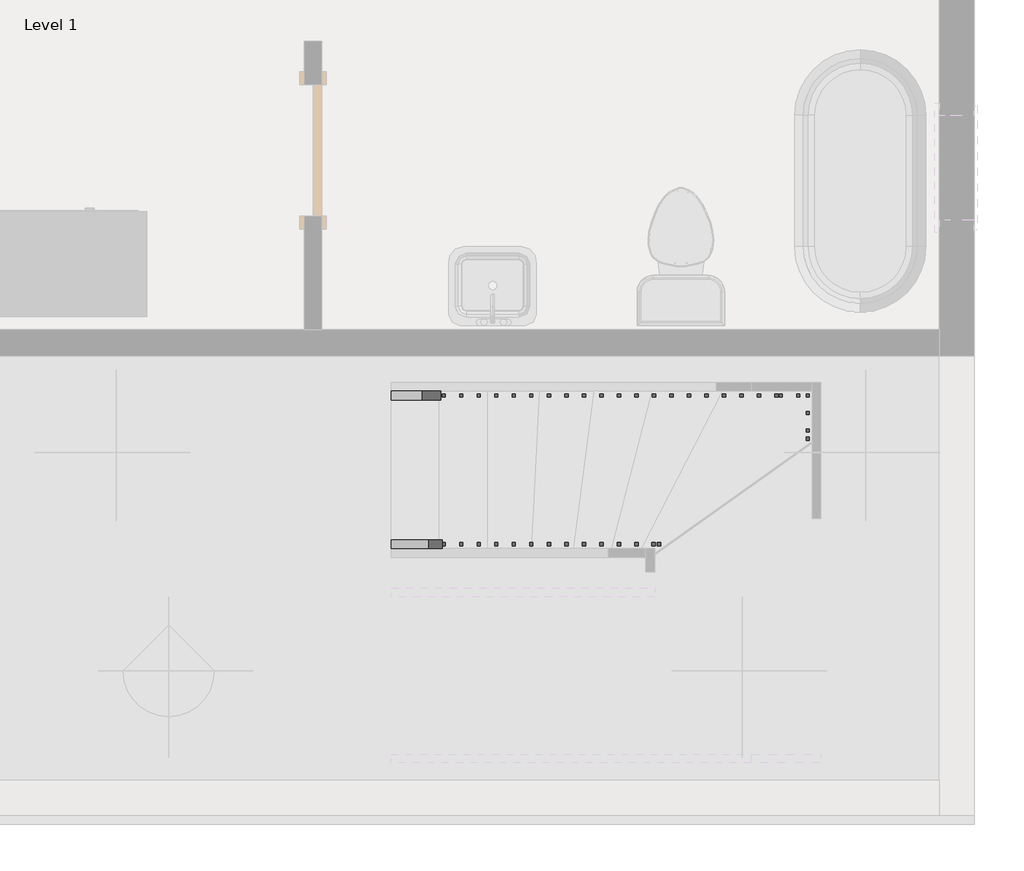
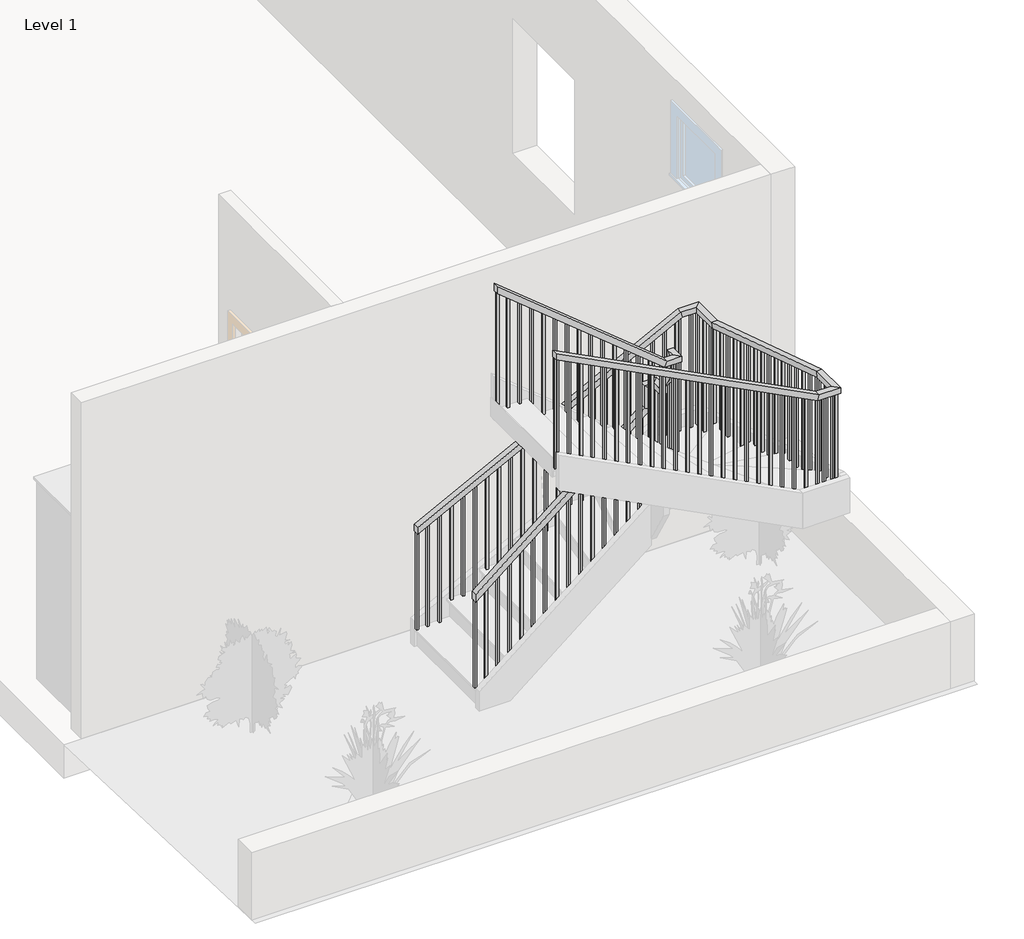
# One storey, part 2 of 3: 2 railings.
"""IFC4 building model written with IfcOpenShell, lengths in millimetres."""

from ifc_helpers import new_model, si_unit, frame, origin, place, context, project, spatial, polyline, outline, extrude, faceted_brep, element, save

model = new_model("IFC4")

# Units and contexts
model_context = context("Model", 3, world=origin())
ifc_project = project(units=[si_unit("LENGTHUNIT", "METRE", prefix="MILLI")], contexts=[model_context])

# Site, building, storey
site = spatial("IfcSite", under=ifc_project)
building = spatial("IfcBuilding", under=site)
storey = spatial("IfcBuildingStorey", under=building, Name="Level 1", Elevation=0.0)

# Railings
placement = place(None, origin())
element("IfcRailing", 1, ObjectType="Handrail - Rectangular", at=placement, inside=storey, context=model_context, shape_type="SolidModel", body=[
    faceted_brep([(3860.8061326, -3864.0192867, 1025.2529681), (3860.8061326, -3864.0192867, 959.7067088), (3860.8061326, -3914.8192867, 959.7067088), (3860.8061326, -3914.8192867, 1025.2529681), (5312.3378245, -3864.0192867, 2208.7848338), (5363.1378245, -3864.0192867, 2184.659247), (5363.1378245, -3914.8192867, 2184.659247), (5312.3378245, -3914.8192867, 2208.7848338), (5312.3378245, -3864.0192867, 2414.6281882), (5363.1378245, -3864.0192867, 2363.8281882), (5363.1378245, -3914.8192867, 2363.8281882), (5312.3378245, -3914.8192867, 2414.6281882), (5439.3378245, -3864.0192867, 2414.6281882), (5439.3378245, -3864.0192867, 2363.8281882), (5388.5378245, -3914.8192867, 2363.8281882), (5388.5378245, -3914.8192867, 2414.6281882), (5439.3378245, -3991.0192867, 2414.6281882), (5439.3378245, -4020.1406205, 2363.8281882), (5388.5378245, -4020.1406205, 2363.8281882), (5388.5378245, -3991.0192867, 2414.6281882), (5439.3378245, -4118.0192867, 2631.5051451), (5439.3378245, -4168.8192867, 2617.7256424), (5388.5378245, -4168.8192867, 2617.7256424), (5388.5378245, -4118.0192867, 2631.5051451), (5439.3378245, -4118.0192867, 2837.3484995), (5439.3378245, -4168.8192867, 2786.5484995), (5388.5378245, -4168.8192867, 2786.5484995), (5388.5378245, -4118.0192867, 2837.3484995), (5439.3378245, -4245.0192867, 2837.3484995), (5439.3378245, -4245.0192867, 2786.5484995), (5388.5378245, -4194.2192867, 2786.5484995), (5388.5378245, -4194.2192867, 2837.3484995), (5312.3378245, -4245.0192867, 2837.3484995), (5294.2524114, -4245.0192867, 2786.5484995), (5294.2524114, -4194.2192867, 2786.5484995), (5312.3378245, -4194.2192867, 2837.3484995), (3860.8061326, -4245.0192867, 4020.8803652), (3860.8061326, -4194.2192867, 4020.8803652), (3860.8061326, -4194.2192867, 3955.3341059), (3860.8061326, -4245.0192867, 3955.3341059)], [[[0, 1, 2, 3]], [[1, 0, 4, 5]], [[2, 1, 5, 6]], [[3, 2, 6, 7]], [[0, 3, 7, 4]], [[5, 4, 8, 9]], [[6, 5, 9, 10]], [[7, 6, 10, 11]], [[4, 7, 11, 8]], [[9, 8, 12, 13]], [[10, 9, 13, 14]], [[11, 10, 14, 15]], [[8, 11, 15, 12]], [[13, 12, 16, 17]], [[14, 13, 17, 18]], [[15, 14, 18, 19]], [[12, 15, 19, 16]], [[17, 16, 20, 21]], [[18, 17, 21, 22]], [[19, 18, 22, 23]], [[16, 19, 23, 20]], [[21, 20, 24, 25]], [[22, 21, 25, 26]], [[23, 22, 26, 27]], [[20, 23, 27, 24]], [[25, 24, 28, 29]], [[26, 25, 29, 30]], [[27, 26, 30, 31]], [[24, 27, 31, 28]], [[29, 28, 32, 33]], [[30, 29, 33, 34]], [[31, 30, 34, 35]], [[28, 31, 35, 32]], [[36, 37, 38, 39]], [[33, 32, 36, 39]], [[34, 33, 39, 38]], [[35, 34, 38, 37]], [[32, 35, 37, 36]]]),
    extrude(outline(polyline([(3866.2231262, 3970.0954681), (3881.7558784, 3951.0454681), (2878.6666667, 3951.0454681), (2878.6666667, 3970.0954681), (3866.2231262, 3970.0954681)])), frame((0.0, -4229.1442867, 0.0), z_axis=(0.0, 1.0, 0.0), x_axis=(0.0, 0.0, 1.0)), (0.0, 0.0, 1.0), 19.05),
    extrude(outline(polyline([(3783.3817813, 4071.6954681), (3798.9145334, 4052.6454681), (2878.6666667, 4052.6454681), (2878.6666667, 4071.6954681), (3783.3817813, 4071.6954681)])), frame((0.0, -4229.1442867, 0.0), z_axis=(0.0, 1.0, 0.0), x_axis=(0.0, 0.0, 1.0)), (0.0, 0.0, 1.0), 19.05),
    extrude(outline(polyline([(3700.5404364, 4173.2954681), (3716.0731885, 4154.2454681), (2709.3333333, 4154.2454681), (2709.3333333, 4173.2954681), (3700.5404364, 4173.2954681)])), frame((0.0, -4229.1442867, 0.0), z_axis=(0.0, 1.0, 0.0), x_axis=(0.0, 0.0, 1.0)), (0.0, 0.0, 1.0), 19.05),
    extrude(outline(polyline([(3617.6990914, 4274.8954681), (3633.2318436, 4255.8454681), (2709.3333333, 4255.8454681), (2709.3333333, 4274.8954681), (3617.6990914, 4274.8954681)])), frame((0.0, -4229.1442867, 0.0), z_axis=(0.0, 1.0, 0.0), x_axis=(0.0, 0.0, 1.0)), (0.0, 0.0, 1.0), 19.05),
    extrude(outline(polyline([(3534.8577465, 4376.4954681), (3550.3904987, 4357.4454681), (2709.3333333, 4357.4454681), (2709.3333333, 4376.4954681), (3534.8577465, 4376.4954681)])), frame((0.0, -4229.1442867, 0.0), z_axis=(0.0, 1.0, 0.0), x_axis=(0.0, 0.0, 1.0)), (0.0, 0.0, 1.0), 19.05),
    extrude(outline(polyline([(3452.0164016, 4478.0954681), (3467.5491538, 4459.0454681), (2540.0, 4459.0454681), (2540.0, 4478.0954681), (3452.0164016, 4478.0954681)])), frame((0.0, -4229.1442867, 0.0), z_axis=(0.0, 1.0, 0.0), x_axis=(0.0, 0.0, 1.0)), (0.0, 0.0, 1.0), 19.05),
    extrude(outline(polyline([(3369.1750567, 4579.6954681), (3384.7078088, 4560.6454681), (2540.0, 4560.6454681), (2540.0, 4579.6954681), (3369.1750567, 4579.6954681)])), frame((0.0, -4229.1442867, 0.0), z_axis=(0.0, 1.0, 0.0), x_axis=(0.0, 0.0, 1.0)), (0.0, 0.0, 1.0), 19.05),
    extrude(outline(polyline([(3286.3337117, 4681.2954681), (3301.8664639, 4662.2454681), (2540.0, 4662.2454681), (2540.0, 4681.2954681), (3286.3337117, 4681.2954681)])), frame((0.0, -4229.1442867, 0.0), z_axis=(0.0, 1.0, 0.0), x_axis=(0.0, 0.0, 1.0)), (0.0, 0.0, 1.0), 19.05),
    extrude(outline(polyline([(3203.4923668, 4782.8954681), (3219.025119, 4763.8454681), (2370.6666667, 4763.8454681), (2370.6666667, 4782.8954681), (3203.4923668, 4782.8954681)])), frame((0.0, -4229.1442867, 0.0), z_axis=(0.0, 1.0, 0.0), x_axis=(0.0, 0.0, 1.0)), (0.0, 0.0, 1.0), 19.05),
    extrude(outline(polyline([(3120.6510219, 4884.4954681), (3136.1837741, 4865.4454681), (2370.6666667, 4865.4454681), (2370.6666667, 4884.4954681), (3120.6510219, 4884.4954681)])), frame((0.0, -4229.1442867, 0.0), z_axis=(0.0, 1.0, 0.0), x_axis=(0.0, 0.0, 1.0)), (0.0, 0.0, 1.0), 19.05),
    extrude(outline(polyline([(3037.809677, 4986.0954681), (3053.3424291, 4967.0454681), (2201.3333333, 4967.0454681), (2201.3333333, 4986.0954681), (3037.809677, 4986.0954681)])), frame((0.0, -4229.1442867, 0.0), z_axis=(0.0, 1.0, 0.0), x_axis=(0.0, 0.0, 1.0)), (0.0, 0.0, 1.0), 19.05),
    extrude(outline(polyline([(2954.9683321, 5087.6954681), (2970.5010842, 5068.6454681), (2201.3333333, 5068.6454681), (2201.3333333, 5087.6954681), (2954.9683321, 5087.6954681)])), frame((0.0, -4229.1442867, 0.0), z_axis=(0.0, 1.0, 0.0), x_axis=(0.0, 0.0, 1.0)), (0.0, 0.0, 1.0), 19.05),
    extrude(outline(polyline([(2872.1269871, 5189.2954681), (2887.6597393, 5170.2454681), (2032.0, 5170.2454681), (2032.0, 5189.2954681), (2872.1269871, 5189.2954681)])), frame((0.0, -4229.1442867, 0.0), z_axis=(0.0, 1.0, 0.0), x_axis=(0.0, 0.0, 1.0)), (0.0, 0.0, 1.0), 19.05),
    extrude(outline(polyline([(2789.2856422, 5290.8954681), (2804.8183944, 5271.8454681), (2032.0, 5271.8454681), (2032.0, 5290.8954681), (2789.2856422, 5290.8954681)])), frame((0.0, -4229.1442867, 0.0), z_axis=(0.0, 1.0, 0.0), x_axis=(0.0, 0.0, 1.0)), (0.0, 0.0, 1.0), 19.05),
    extrude(outline(polyline([(-4116.9301904, 2529.115018), (-4097.8801904, 2496.5834745), (-4097.8801904, 1524.0), (-4116.9301904, 1524.0), (-4116.9301904, 2529.115018)])), frame((5404.4128245, 0.0, 0.0), z_axis=(1.0, 0.0, 0.0), x_axis=(0.0, 1.0, 0.0)), (0.0, 0.0, 1.0), 19.05),
    extrude(outline(polyline([(-4015.3301904, 2355.6134525), (-3996.2801904, 2323.0819089), (-3996.2801904, 1524.0), (-4015.3301904, 1524.0), (-4015.3301904, 2355.6134525)])), frame((5404.4128245, 0.0, 0.0), z_axis=(1.0, 0.0, 0.0), x_axis=(0.0, 1.0, 0.0)), (0.0, 0.0, 1.0), 19.05),
    extrude(outline(polyline([(2127.2519138, 5292.7311326), (2111.7191617, 5273.6811326), (1016.0, 5273.6811326), (1016.0, 5292.7311326), (2127.2519138, 5292.7311326)])), frame((0.0, -3898.9442867, 0.0), z_axis=(0.0, 1.0, 0.0), x_axis=(0.0, 0.0, 1.0)), (0.0, 0.0, 1.0), 19.05),
    extrude(outline(polyline([(2044.4105689, 5191.1311326), (2028.8778167, 5172.0811326), (1016.0, 5172.0811326), (1016.0, 5191.1311326), (2044.4105689, 5191.1311326)])), frame((0.0, -3898.9442867, 0.0), z_axis=(0.0, 1.0, 0.0), x_axis=(0.0, 0.0, 1.0)), (0.0, 0.0, 1.0), 19.05),
    extrude(outline(polyline([(1961.569224, 5089.5311326), (1946.0364718, 5070.4811326), (846.6666667, 5070.4811326), (846.6666667, 5089.5311326), (1961.569224, 5089.5311326)])), frame((0.0, -3898.9442867, 0.0), z_axis=(0.0, 1.0, 0.0), x_axis=(0.0, 0.0, 1.0)), (0.0, 0.0, 1.0), 19.05),
    extrude(outline(polyline([(1878.7278791, 4987.9311326), (1863.1951269, 4968.8811326), (846.6666667, 4968.8811326), (846.6666667, 4987.9311326), (1878.7278791, 4987.9311326)])), frame((0.0, -3898.9442867, 0.0), z_axis=(0.0, 1.0, 0.0), x_axis=(0.0, 0.0, 1.0)), (0.0, 0.0, 1.0), 19.05),
    extrude(outline(polyline([(1795.8865341, 4886.3311326), (1780.353782, 4867.2811326), (677.3333333, 4867.2811326), (677.3333333, 4886.3311326), (1795.8865341, 4886.3311326)])), frame((0.0, -3898.9442867, 0.0), z_axis=(0.0, 1.0, 0.0), x_axis=(0.0, 0.0, 1.0)), (0.0, 0.0, 1.0), 19.05),
    extrude(outline(polyline([(1713.0451892, 4784.7311326), (1697.5124371, 4765.6811326), (677.3333333, 4765.6811326), (677.3333333, 4784.7311326), (1713.0451892, 4784.7311326)])), frame((0.0, -3898.9442867, 0.0), z_axis=(0.0, 1.0, 0.0), x_axis=(0.0, 0.0, 1.0)), (0.0, 0.0, 1.0), 19.05),
    extrude(outline(polyline([(1630.2038443, 4683.1311326), (1614.6710921, 4664.0811326), (508.0, 4664.0811326), (508.0, 4683.1311326), (1630.2038443, 4683.1311326)])), frame((0.0, -3898.9442867, 0.0), z_axis=(0.0, 1.0, 0.0), x_axis=(0.0, 0.0, 1.0)), (0.0, 0.0, 1.0), 19.05),
    extrude(outline(polyline([(1547.3624994, 4581.5311326), (1531.8297472, 4562.4811326), (508.0, 4562.4811326), (508.0, 4581.5311326), (1547.3624994, 4581.5311326)])), frame((0.0, -3898.9442867, 0.0), z_axis=(0.0, 1.0, 0.0), x_axis=(0.0, 0.0, 1.0)), (0.0, 0.0, 1.0), 19.05),
    extrude(outline(polyline([(1464.5211545, 4479.9311326), (1448.9884023, 4460.8811326), (508.0, 4460.8811326), (508.0, 4479.9311326), (1464.5211545, 4479.9311326)])), frame((0.0, -3898.9442867, 0.0), z_axis=(0.0, 1.0, 0.0), x_axis=(0.0, 0.0, 1.0)), (0.0, 0.0, 1.0), 19.05),
    extrude(outline(polyline([(1381.6798095, 4378.3311326), (1366.1470574, 4359.2811326), (338.6666667, 4359.2811326), (338.6666667, 4378.3311326), (1381.6798095, 4378.3311326)])), frame((0.0, -3898.9442867, 0.0), z_axis=(0.0, 1.0, 0.0), x_axis=(0.0, 0.0, 1.0)), (0.0, 0.0, 1.0), 19.05),
    extrude(outline(polyline([(1298.8384646, 4276.7311326), (1283.3057124, 4257.6811326), (338.6666667, 4257.6811326), (338.6666667, 4276.7311326), (1298.8384646, 4276.7311326)])), frame((0.0, -3898.9442867, 0.0), z_axis=(0.0, 1.0, 0.0), x_axis=(0.0, 0.0, 1.0)), (0.0, 0.0, 1.0), 19.05),
    extrude(outline(polyline([(1215.9971197, 4175.1311326), (1200.4643675, 4156.0811326), (338.6666667, 4156.0811326), (338.6666667, 4175.1311326), (1215.9971197, 4175.1311326)])), frame((0.0, -3898.9442867, 0.0), z_axis=(0.0, 1.0, 0.0), x_axis=(0.0, 0.0, 1.0)), (0.0, 0.0, 1.0), 19.05),
    extrude(outline(polyline([(1133.1557748, 4073.5311326), (1117.6230226, 4054.4811326), (169.3333333, 4054.4811326), (169.3333333, 4073.5311326), (1133.1557748, 4073.5311326)])), frame((0.0, -3898.9442867, 0.0), z_axis=(0.0, 1.0, 0.0), x_axis=(0.0, 0.0, 1.0)), (0.0, 0.0, 1.0), 19.05),
    extrude(outline(polyline([(1050.3144298, 3971.9311326), (1034.7816777, 3952.8811326), (169.3333333, 3952.8811326), (169.3333333, 3971.9311326), (1050.3144298, 3971.9311326)])), frame((0.0, -3898.9442867, 0.0), z_axis=(0.0, 1.0, 0.0), x_axis=(0.0, 0.0, 1.0)), (0.0, 0.0, 1.0), 19.05),
    extrude(outline(polyline([(5392.4954681, -4210.0942867), (5392.4954681, -4229.1442867), (5373.4454681, -4229.1442867), (5373.4454681, -4210.0942867), (5392.4954681, -4210.0942867)])), frame((0.0, 0.0, 1862.6666667), z_axis=(0.0, 0.0, 1.0), x_axis=(1.0, 0.0, 0.0)), (0.0, 0.0, 1.0), 923.8818329),
    extrude(outline(polyline([(5404.4128245, -4210.0942867), (5423.4628245, -4210.0942867), (5423.4628245, -4229.1442867), (5404.4128245, -4229.1442867), (5404.4128245, -4210.0942867)])), frame((0.0, 0.0, 1862.6666667), z_axis=(0.0, 0.0, 1.0), x_axis=(1.0, 0.0, 0.0)), (0.0, 0.0, 1.0), 923.8818329),
    extrude(outline(polyline([(5404.4128245, -4195.3083829), (5423.4628245, -4195.3083829), (5423.4628245, -4214.3583829), (5404.4128245, -4214.3583829), (5404.4128245, -4195.3083829)])), frame((0.0, 0.0, 1693.3333333), z_axis=(0.0, 0.0, 1.0), x_axis=(1.0, 0.0, 0.0)), (0.0, 0.0, 1.0), 1093.2151662),
    extrude(outline(polyline([(5404.4128245, -3894.6801904), (5423.4628245, -3894.6801904), (5423.4628245, -3913.7301904), (5404.4128245, -3913.7301904), (5404.4128245, -3894.6801904)])), frame((0.0, 0.0, 1354.6666667), z_axis=(0.0, 0.0, 1.0), x_axis=(1.0, 0.0, 0.0)), (0.0, 0.0, 1.0), 1009.1615215),
    extrude(outline(polyline([(5404.4128245, -3898.9442867), (5404.4128245, -3879.8942867), (5423.4628245, -3879.8942867), (5423.4628245, -3898.9442867), (5404.4128245, -3898.9442867)])), frame((0.0, 0.0, 1185.3333333), z_axis=(0.0, 0.0, 1.0), x_axis=(1.0, 0.0, 0.0)), (0.0, 0.0, 1.0), 1178.4948549),
    extrude(outline(polyline([(5373.4454681, -3898.9442867), (5373.4454681, -3879.8942867), (5392.4954681, -3879.8942867), (5392.4954681, -3898.9442867), (5373.4454681, -3898.9442867)])), frame((0.0, 0.0, 1185.3333333), z_axis=(0.0, 0.0, 1.0), x_axis=(1.0, 0.0, 0.0)), (0.0, 0.0, 1.0), 1178.4948549),
    extrude(outline(polyline([(3939.8013537, 3879.8561326), (3955.3341059, 3860.8061326), (2878.6666667, 3860.8061326), (2878.6666667, 3879.8561326), (3939.8013537, 3879.8561326)])), frame((0.0, -4229.1442867, 0.0), z_axis=(0.0, 1.0, 0.0), x_axis=(0.0, 0.0, 1.0)), (0.0, 0.0, 1.0), 19.05),
    extrude(outline(polyline([(975.239461, 3879.8561326), (959.7067088, 3860.8061326), (169.3333333, 3860.8061326), (169.3333333, 3879.8561326), (975.239461, 3879.8561326)])), frame((0.0, -3898.9442867, 0.0), z_axis=(0.0, 1.0, 0.0), x_axis=(0.0, 0.0, 1.0)), (0.0, 0.0, 1.0), 19.05),
])
element("IfcRailing", 2, ObjectType="Handrail - Rectangular", at=placement, inside=storey, context=model_context, shape_type="SolidModel", body=[
    faceted_brep([(3860.8061326, -3000.4192867, 1109.0771751), (3860.8061326, -3000.4192867, 1051.9280057), (3860.8061326, -3051.2192867, 1051.9280057), (3860.8061326, -3051.2192867, 1109.0771751), (6120.7879891, -3000.4192867, 2273.7644996), (6133.1080404, -3000.4192867, 2222.9644996), (6133.1080404, -3051.2192867, 2222.9644996), (6120.7879891, -3051.2192867, 2273.7644996), (6302.9378245, -3000.4192867, 2273.7644996), (6302.9378245, -3000.4192867, 2222.9644996), (6252.1378245, -3051.2192867, 2222.9644996), (6252.1378245, -3051.2192867, 2273.7644996), (6302.9378245, -3277.5732393, 2273.7644996), (6302.9378245, -3285.5238154, 2222.9644996), (6252.1378245, -3285.5238154, 2222.9644996), (6252.1378245, -3277.5732393, 2273.7644996), (6302.9378245, -4831.4653341, 2772.3688337), (6302.9378245, -4839.4159102, 2721.5688337), (6252.1378245, -4839.4159102, 2721.5688337), (6252.1378245, -4831.4653341, 2772.3688337), (6302.9378245, -5108.6192867, 2772.3688337), (6302.9378245, -5108.6192867, 2721.5688337), (6252.1378245, -5057.8192867, 2721.5688337), (6252.1378245, -5057.8192867, 2772.3688337), (6120.7879891, -5108.6192867, 2772.3688337), (6108.4679378, -5108.6192867, 2721.5688337), (6108.4679378, -5057.8192867, 2721.5688337), (6120.7879891, -5057.8192867, 2772.3688337), (3860.8061326, -5108.6192867, 3937.0561582), (3860.8061326, -5057.8192867, 3937.0561582), (3860.8061326, -5057.8192867, 3879.9069889), (3860.8061326, -5108.6192867, 3879.9069889)], [[[0, 1, 2, 3]], [[1, 0, 4, 5]], [[2, 1, 5, 6]], [[3, 2, 6, 7]], [[0, 3, 7, 4]], [[5, 4, 8, 9]], [[6, 5, 9, 10]], [[7, 6, 10, 11]], [[4, 7, 11, 8]], [[9, 8, 12, 13]], [[10, 9, 13, 14]], [[11, 10, 14, 15]], [[8, 11, 15, 12]], [[13, 12, 16, 17]], [[14, 13, 17, 18]], [[15, 14, 18, 19]], [[12, 15, 19, 16]], [[17, 16, 20, 21]], [[18, 17, 21, 22]], [[19, 18, 22, 23]], [[16, 19, 23, 20]], [[21, 20, 24, 25]], [[22, 21, 25, 26]], [[23, 22, 26, 27]], [[20, 23, 27, 24]], [[28, 29, 30, 31]], [[25, 24, 28, 31]], [[26, 25, 31, 30]], [[27, 26, 30, 29]], [[24, 27, 29, 28]]]),
    extrude(outline(polyline([(3872.0443296, 3876.0629891), (2878.6666667, 3876.0629891), (2878.6666667, 3895.1129891), (3862.2268642, 3895.1129891), (3872.0443296, 3876.0629891)])), frame((0.0, -5092.7442867, 0.0), z_axis=(0.0, 1.0, 0.0), x_axis=(0.0, 0.0, 1.0)), (0.0, 0.0, 1.0), 19.05),
    extrude(outline(polyline([(3819.6845145, 3977.6629891), (2878.6666667, 3977.6629891), (2878.6666667, 3996.7129891), (3809.8670491, 3996.7129891), (3819.6845145, 3977.6629891)])), frame((0.0, -5092.7442867, 0.0), z_axis=(0.0, 1.0, 0.0), x_axis=(0.0, 0.0, 1.0)), (0.0, 0.0, 1.0), 19.05),
    extrude(outline(polyline([(3767.3246993, 4079.2629891), (2878.6666667, 4079.2629891), (2878.6666667, 4098.3129891), (3757.507234, 4098.3129891), (3767.3246993, 4079.2629891)])), frame((0.0, -5092.7442867, 0.0), z_axis=(0.0, 1.0, 0.0), x_axis=(0.0, 0.0, 1.0)), (0.0, 0.0, 1.0), 19.05),
    extrude(outline(polyline([(3714.9648842, 4180.8629891), (2709.3333333, 4180.8629891), (2709.3333333, 4199.9129891), (3705.1474189, 4199.9129891), (3714.9648842, 4180.8629891)])), frame((0.0, -5092.7442867, 0.0), z_axis=(0.0, 1.0, 0.0), x_axis=(0.0, 0.0, 1.0)), (0.0, 0.0, 1.0), 19.05),
    extrude(outline(polyline([(3662.6050691, 4282.4629891), (2709.3333333, 4282.4629891), (2709.3333333, 4301.5129891), (3652.7876038, 4301.5129891), (3662.6050691, 4282.4629891)])), frame((0.0, -5092.7442867, 0.0), z_axis=(0.0, 1.0, 0.0), x_axis=(0.0, 0.0, 1.0)), (0.0, 0.0, 1.0), 19.05),
    extrude(outline(polyline([(3610.245254, 4384.0629891), (2709.3333333, 4384.0629891), (2709.3333333, 4403.1129891), (3600.4277887, 4403.1129891), (3610.245254, 4384.0629891)])), frame((0.0, -5092.7442867, 0.0), z_axis=(0.0, 1.0, 0.0), x_axis=(0.0, 0.0, 1.0)), (0.0, 0.0, 1.0), 19.05),
    extrude(outline(polyline([(3557.8854389, 4485.6629891), (2540.0, 4485.6629891), (2540.0, 4504.7129891), (3548.0679735, 4504.7129891), (3557.8854389, 4485.6629891)])), frame((0.0, -5092.7442867, 0.0), z_axis=(0.0, 1.0, 0.0), x_axis=(0.0, 0.0, 1.0)), (0.0, 0.0, 1.0), 19.05),
    extrude(outline(polyline([(3505.5256238, 4587.2629891), (2540.0, 4587.2629891), (2540.0, 4606.3129891), (3495.7081584, 4606.3129891), (3505.5256238, 4587.2629891)])), frame((0.0, -5092.7442867, 0.0), z_axis=(0.0, 1.0, 0.0), x_axis=(0.0, 0.0, 1.0)), (0.0, 0.0, 1.0), 19.05),
    extrude(outline(polyline([(3453.1658086, 4688.8629891), (2540.0, 4688.8629891), (2540.0, 4707.9129891), (3443.3483433, 4707.9129891), (3453.1658086, 4688.8629891)])), frame((0.0, -5092.7442867, 0.0), z_axis=(0.0, 1.0, 0.0), x_axis=(0.0, 0.0, 1.0)), (0.0, 0.0, 1.0), 19.05),
    extrude(outline(polyline([(3400.8059935, 4790.4629891), (2370.6666667, 4790.4629891), (2370.6666667, 4809.5129891), (3390.9885282, 4809.5129891), (3400.8059935, 4790.4629891)])), frame((0.0, -5092.7442867, 0.0), z_axis=(0.0, 1.0, 0.0), x_axis=(0.0, 0.0, 1.0)), (0.0, 0.0, 1.0), 19.05),
    extrude(outline(polyline([(3348.4461784, 4892.0629891), (2370.6666667, 4892.0629891), (2370.6666667, 4911.1129891), (3338.6287131, 4911.1129891), (3348.4461784, 4892.0629891)])), frame((0.0, -5092.7442867, 0.0), z_axis=(0.0, 1.0, 0.0), x_axis=(0.0, 0.0, 1.0)), (0.0, 0.0, 1.0), 19.05),
    extrude(outline(polyline([(3296.0863633, 4993.6629891), (2370.6666667, 4993.6629891), (2370.6666667, 5012.7129891), (3286.268898, 5012.7129891), (3296.0863633, 4993.6629891)])), frame((0.0, -5092.7442867, 0.0), z_axis=(0.0, 1.0, 0.0), x_axis=(0.0, 0.0, 1.0)), (0.0, 0.0, 1.0), 19.05),
    extrude(outline(polyline([(3243.7265482, 5095.2629891), (2201.3333333, 5095.2629891), (2201.3333333, 5114.3129891), (3233.9090828, 5114.3129891), (3243.7265482, 5095.2629891)])), frame((0.0, -5092.7442867, 0.0), z_axis=(0.0, 1.0, 0.0), x_axis=(0.0, 0.0, 1.0)), (0.0, 0.0, 1.0), 19.05),
    extrude(outline(polyline([(3191.3667331, 5196.8629891), (2201.3333333, 5196.8629891), (2201.3333333, 5215.9129891), (3181.5492677, 5215.9129891), (3191.3667331, 5196.8629891)])), frame((0.0, -5092.7442867, 0.0), z_axis=(0.0, 1.0, 0.0), x_axis=(0.0, 0.0, 1.0)), (0.0, 0.0, 1.0), 19.05),
    extrude(outline(polyline([(3139.0069179, 5298.4629891), (2201.3333333, 5298.4629891), (2201.3333333, 5317.5129891), (3129.1894526, 5317.5129891), (3139.0069179, 5298.4629891)])), frame((0.0, -5092.7442867, 0.0), z_axis=(0.0, 1.0, 0.0), x_axis=(0.0, 0.0, 1.0)), (0.0, 0.0, 1.0), 19.05),
    extrude(outline(polyline([(3086.6471028, 5400.0629891), (2032.0, 5400.0629891), (2032.0, 5419.1129891), (3076.8296375, 5419.1129891), (3086.6471028, 5400.0629891)])), frame((0.0, -5092.7442867, 0.0), z_axis=(0.0, 1.0, 0.0), x_axis=(0.0, 0.0, 1.0)), (0.0, 0.0, 1.0), 19.05),
    extrude(outline(polyline([(3034.2872877, 5501.6629891), (2032.0, 5501.6629891), (2032.0, 5520.7129891), (3024.4698224, 5520.7129891), (3034.2872877, 5501.6629891)])), frame((0.0, -5092.7442867, 0.0), z_axis=(0.0, 1.0, 0.0), x_axis=(0.0, 0.0, 1.0)), (0.0, 0.0, 1.0), 19.05),
    extrude(outline(polyline([(2981.9274726, 5603.2629891), (2032.0, 5603.2629891), (2032.0, 5622.3129891), (2972.1100073, 5622.3129891), (2981.9274726, 5603.2629891)])), frame((0.0, -5092.7442867, 0.0), z_axis=(0.0, 1.0, 0.0), x_axis=(0.0, 0.0, 1.0)), (0.0, 0.0, 1.0), 19.05),
    extrude(outline(polyline([(2929.5676575, 5704.8629891), (2032.0, 5704.8629891), (2032.0, 5723.9129891), (2919.7501921, 5723.9129891), (2929.5676575, 5704.8629891)])), frame((0.0, -5092.7442867, 0.0), z_axis=(0.0, 1.0, 0.0), x_axis=(0.0, 0.0, 1.0)), (0.0, 0.0, 1.0), 19.05),
    extrude(outline(polyline([(2877.2078424, 5806.4629891), (1862.6666667, 5806.4629891), (1862.6666667, 5825.5129891), (2867.390377, 5825.5129891), (2877.2078424, 5806.4629891)])), frame((0.0, -5092.7442867, 0.0), z_axis=(0.0, 1.0, 0.0), x_axis=(0.0, 0.0, 1.0)), (0.0, 0.0, 1.0), 19.05),
    extrude(outline(polyline([(2824.8480272, 5908.0629891), (1862.6666667, 5908.0629891), (1862.6666667, 5927.1129891), (2815.0305619, 5927.1129891), (2824.8480272, 5908.0629891)])), frame((0.0, -5092.7442867, 0.0), z_axis=(0.0, 1.0, 0.0), x_axis=(0.0, 0.0, 1.0)), (0.0, 0.0, 1.0), 19.05),
    extrude(outline(polyline([(2772.4882121, 6009.6629891), (1862.6666667, 6009.6629891), (1862.6666667, 6028.7129891), (2762.6707468, 6028.7129891), (2772.4882121, 6009.6629891)])), frame((0.0, -5092.7442867, 0.0), z_axis=(0.0, 1.0, 0.0), x_axis=(0.0, 0.0, 1.0)), (0.0, 0.0, 1.0), 19.05),
    extrude(outline(polyline([(6185.4628245, -5092.7442867), (6166.4128245, -5092.7442867), (6166.4128245, -5073.6942867), (6185.4628245, -5073.6942867), (6185.4628245, -5092.7442867)])), frame((0.0, 0.0, 1862.6666667), z_axis=(0.0, 0.0, 1.0), x_axis=(1.0, 0.0, 0.0)), (0.0, 0.0, 1.0), 858.902167),
    extrude(outline(polyline([(6287.0628245, -5025.1403341), (6287.0628245, -5044.1903341), (6268.0128245, -5044.1903341), (6268.0128245, -5025.1403341), (6287.0628245, -5025.1403341)])), frame((0.0, 0.0, 1862.6666667), z_axis=(0.0, 0.0, 1.0), x_axis=(1.0, 0.0, 0.0)), (0.0, 0.0, 1.0), 858.902167),
    extrude(outline(polyline([(6287.0628245, -4923.5403341), (6287.0628245, -4942.5903341), (6268.0128245, -4942.5903341), (6268.0128245, -4923.5403341), (6287.0628245, -4923.5403341)])), frame((0.0, 0.0, 1862.6666667), z_axis=(0.0, 0.0, 1.0), x_axis=(1.0, 0.0, 0.0)), (0.0, 0.0, 1.0), 858.902167),
    extrude(outline(polyline([(-4792.0482393, 2706.3697564), (-4792.0482393, 1693.3333333), (-4811.0982393, 1693.3333333), (-4811.0982393, 2712.4824155), (-4792.0482393, 2706.3697564)])), frame((6268.0128245, 0.0, 0.0), z_axis=(1.0, 0.0, 0.0), x_axis=(0.0, 1.0, 0.0)), (0.0, 0.0, 1.0), 19.05),
    extrude(outline(polyline([(-4690.4482393, 2673.7689082), (-4690.4482393, 1693.3333333), (-4709.4982393, 1693.3333333), (-4709.4982393, 2679.8815673), (-4690.4482393, 2673.7689082)])), frame((6268.0128245, 0.0, 0.0), z_axis=(1.0, 0.0, 0.0), x_axis=(0.0, 1.0, 0.0)), (0.0, 0.0, 1.0), 19.05),
    extrude(outline(polyline([(-4588.8482393, 2641.16806), (-4588.8482393, 1693.3333333), (-4607.8982393, 1693.3333333), (-4607.8982393, 2647.280719), (-4588.8482393, 2641.16806)])), frame((6268.0128245, 0.0, 0.0), z_axis=(1.0, 0.0, 0.0), x_axis=(0.0, 1.0, 0.0)), (0.0, 0.0, 1.0), 19.05),
    extrude(outline(polyline([(-4487.2482393, 2608.5672118), (-4487.2482393, 1693.3333333), (-4506.2982393, 1693.3333333), (-4506.2982393, 2614.6798708), (-4487.2482393, 2608.5672118)])), frame((6268.0128245, 0.0, 0.0), z_axis=(1.0, 0.0, 0.0), x_axis=(0.0, 1.0, 0.0)), (0.0, 0.0, 1.0), 19.05),
    extrude(outline(polyline([(-4385.6482393, 2575.9663635), (-4385.6482393, 1693.3333333), (-4404.6982393, 1693.3333333), (-4404.6982393, 2582.0790226), (-4385.6482393, 2575.9663635)])), frame((6268.0128245, 0.0, 0.0), z_axis=(1.0, 0.0, 0.0), x_axis=(0.0, 1.0, 0.0)), (0.0, 0.0, 1.0), 19.05),
    extrude(outline(polyline([(-4284.0482393, 2543.3655153), (-4284.0482393, 1693.3333333), (-4303.0982393, 1693.3333333), (-4303.0982393, 2549.4781744), (-4284.0482393, 2543.3655153)])), frame((6268.0128245, 0.0, 0.0), z_axis=(1.0, 0.0, 0.0), x_axis=(0.0, 1.0, 0.0)), (0.0, 0.0, 1.0), 19.05),
    extrude(outline(polyline([(-4182.4482393, 2510.7646671), (-4182.4482393, 1524.0), (-4201.4982393, 1524.0), (-4201.4982393, 2516.8773261), (-4182.4482393, 2510.7646671)])), frame((6268.0128245, 0.0, 0.0), z_axis=(1.0, 0.0, 0.0), x_axis=(0.0, 1.0, 0.0)), (0.0, 0.0, 1.0), 19.05),
    extrude(outline(polyline([(-4080.8482393, 2478.1638189), (-4080.8482393, 1524.0), (-4099.8982393, 1524.0), (-4099.8982393, 2484.2764779), (-4080.8482393, 2478.1638189)])), frame((6268.0128245, 0.0, 0.0), z_axis=(1.0, 0.0, 0.0), x_axis=(0.0, 1.0, 0.0)), (0.0, 0.0, 1.0), 19.05),
    extrude(outline(polyline([(-3979.2482393, 2445.5629706), (-3979.2482393, 1524.0), (-3998.2982393, 1524.0), (-3998.2982393, 2451.6756297), (-3979.2482393, 2445.5629706)])), frame((6268.0128245, 0.0, 0.0), z_axis=(1.0, 0.0, 0.0), x_axis=(0.0, 1.0, 0.0)), (0.0, 0.0, 1.0), 19.05),
    extrude(outline(polyline([(-3877.6482393, 2412.9621224), (-3877.6482393, 1524.0), (-3896.6982393, 1524.0), (-3896.6982393, 2419.0747814), (-3877.6482393, 2412.9621224)])), frame((6268.0128245, 0.0, 0.0), z_axis=(1.0, 0.0, 0.0), x_axis=(0.0, 1.0, 0.0)), (0.0, 0.0, 1.0), 19.05),
    extrude(outline(polyline([(-3776.0482393, 2380.3612742), (-3776.0482393, 1354.6666667), (-3795.0982393, 1354.6666667), (-3795.0982393, 2386.4739332), (-3776.0482393, 2380.3612742)])), frame((6268.0128245, 0.0, 0.0), z_axis=(1.0, 0.0, 0.0), x_axis=(0.0, 1.0, 0.0)), (0.0, 0.0, 1.0), 19.05),
    extrude(outline(polyline([(-3674.4482393, 2347.7604259), (-3674.4482393, 1354.6666667), (-3693.4982393, 1354.6666667), (-3693.4982393, 2353.873085), (-3674.4482393, 2347.7604259)])), frame((6268.0128245, 0.0, 0.0), z_axis=(1.0, 0.0, 0.0), x_axis=(0.0, 1.0, 0.0)), (0.0, 0.0, 1.0), 19.05),
    extrude(outline(polyline([(-3572.8482393, 2315.1595777), (-3572.8482393, 1354.6666667), (-3591.8982393, 1354.6666667), (-3591.8982393, 2321.2722368), (-3572.8482393, 2315.1595777)])), frame((6268.0128245, 0.0, 0.0), z_axis=(1.0, 0.0, 0.0), x_axis=(0.0, 1.0, 0.0)), (0.0, 0.0, 1.0), 19.05),
    extrude(outline(polyline([(-3471.2482393, 2282.5587295), (-3471.2482393, 1354.6666667), (-3490.2982393, 1354.6666667), (-3490.2982393, 2288.6713885), (-3471.2482393, 2282.5587295)])), frame((6268.0128245, 0.0, 0.0), z_axis=(1.0, 0.0, 0.0), x_axis=(0.0, 1.0, 0.0)), (0.0, 0.0, 1.0), 19.05),
    extrude(outline(polyline([(-3369.6482393, 2249.9578813), (-3369.6482393, 1354.6666667), (-3388.6982393, 1354.6666667), (-3388.6982393, 2256.0705403), (-3369.6482393, 2249.9578813)])), frame((6268.0128245, 0.0, 0.0), z_axis=(1.0, 0.0, 0.0), x_axis=(0.0, 1.0, 0.0)), (0.0, 0.0, 1.0), 19.05),
    extrude(outline(polyline([(6287.0628245, -3219.4942867), (6287.0628245, -3238.5442867), (6268.0128245, -3238.5442867), (6268.0128245, -3219.4942867), (6287.0628245, -3219.4942867)])), frame((0.0, 0.0, 1185.3333333), z_axis=(0.0, 0.0, 1.0), x_axis=(1.0, 0.0, 0.0)), (0.0, 0.0, 1.0), 1037.6311663),
    extrude(outline(polyline([(6287.0628245, -3117.8942867), (6287.0628245, -3136.9442867), (6268.0128245, -3136.9442867), (6268.0128245, -3117.8942867), (6287.0628245, -3117.8942867)])), frame((0.0, 0.0, 1185.3333333), z_axis=(0.0, 0.0, 1.0), x_axis=(1.0, 0.0, 0.0)), (0.0, 0.0, 1.0), 1037.6311663),
    extrude(outline(polyline([(6212.8629891, -3016.2942867), (6231.9129891, -3016.2942867), (6231.9129891, -3035.3442867), (6212.8629891, -3035.3442867), (6212.8629891, -3016.2942867)])), frame((0.0, 0.0, 1185.3333333), z_axis=(0.0, 0.0, 1.0), x_axis=(1.0, 0.0, 0.0)), (0.0, 0.0, 1.0), 1037.6311663),
    extrude(outline(polyline([(2198.9352056, 6086.4811326), (1185.3333333, 6086.4811326), (1185.3333333, 6105.5311326), (2208.752671, 6105.5311326), (2198.9352056, 6086.4811326)])), frame((0.0, -3035.3442867, 0.0), z_axis=(0.0, 1.0, 0.0), x_axis=(0.0, 0.0, 1.0)), (0.0, 0.0, 1.0), 19.05),
    extrude(outline(polyline([(2146.5753905, 5984.8811326), (1185.3333333, 5984.8811326), (1185.3333333, 6003.9311326), (2156.3928558, 6003.9311326), (2146.5753905, 5984.8811326)])), frame((0.0, -3035.3442867, 0.0), z_axis=(0.0, 1.0, 0.0), x_axis=(0.0, 0.0, 1.0)), (0.0, 0.0, 1.0), 19.05),
    extrude(outline(polyline([(2094.2155754, 5883.2811326), (1185.3333333, 5883.2811326), (1185.3333333, 5902.3311326), (2104.0330407, 5902.3311326), (2094.2155754, 5883.2811326)])), frame((0.0, -3035.3442867, 0.0), z_axis=(0.0, 1.0, 0.0), x_axis=(0.0, 0.0, 1.0)), (0.0, 0.0, 1.0), 19.05),
    extrude(outline(polyline([(2041.8557603, 5781.6811326), (1185.3333333, 5781.6811326), (1185.3333333, 5800.7311326), (2051.6732256, 5800.7311326), (2041.8557603, 5781.6811326)])), frame((0.0, -3035.3442867, 0.0), z_axis=(0.0, 1.0, 0.0), x_axis=(0.0, 0.0, 1.0)), (0.0, 0.0, 1.0), 19.05),
    extrude(outline(polyline([(1989.4959452, 5680.0811326), (1016.0, 5680.0811326), (1016.0, 5699.1311326), (1999.3134105, 5699.1311326), (1989.4959452, 5680.0811326)])), frame((0.0, -3035.3442867, 0.0), z_axis=(0.0, 1.0, 0.0), x_axis=(0.0, 0.0, 1.0)), (0.0, 0.0, 1.0), 19.05),
    extrude(outline(polyline([(1937.13613, 5578.4811326), (1016.0, 5578.4811326), (1016.0, 5597.5311326), (1946.9535954, 5597.5311326), (1937.13613, 5578.4811326)])), frame((0.0, -3035.3442867, 0.0), z_axis=(0.0, 1.0, 0.0), x_axis=(0.0, 0.0, 1.0)), (0.0, 0.0, 1.0), 19.05),
    extrude(outline(polyline([(1884.7763149, 5476.8811326), (1016.0, 5476.8811326), (1016.0, 5495.9311326), (1894.5937803, 5495.9311326), (1884.7763149, 5476.8811326)])), frame((0.0, -3035.3442867, 0.0), z_axis=(0.0, 1.0, 0.0), x_axis=(0.0, 0.0, 1.0)), (0.0, 0.0, 1.0), 19.05),
    extrude(outline(polyline([(1832.4164998, 5375.2811326), (1016.0, 5375.2811326), (1016.0, 5394.3311326), (1842.2339651, 5394.3311326), (1832.4164998, 5375.2811326)])), frame((0.0, -3035.3442867, 0.0), z_axis=(0.0, 1.0, 0.0), x_axis=(0.0, 0.0, 1.0)), (0.0, 0.0, 1.0), 19.05),
    extrude(outline(polyline([(1780.0566847, 5273.6811326), (846.6666667, 5273.6811326), (846.6666667, 5292.7311326), (1789.87415, 5292.7311326), (1780.0566847, 5273.6811326)])), frame((0.0, -3035.3442867, 0.0), z_axis=(0.0, 1.0, 0.0), x_axis=(0.0, 0.0, 1.0)), (0.0, 0.0, 1.0), 19.05),
    extrude(outline(polyline([(1727.6968696, 5172.0811326), (846.6666667, 5172.0811326), (846.6666667, 5191.1311326), (1737.5143349, 5191.1311326), (1727.6968696, 5172.0811326)])), frame((0.0, -3035.3442867, 0.0), z_axis=(0.0, 1.0, 0.0), x_axis=(0.0, 0.0, 1.0)), (0.0, 0.0, 1.0), 19.05),
    extrude(outline(polyline([(1675.3370545, 5070.4811326), (846.6666667, 5070.4811326), (846.6666667, 5089.5311326), (1685.1545198, 5089.5311326), (1675.3370545, 5070.4811326)])), frame((0.0, -3035.3442867, 0.0), z_axis=(0.0, 1.0, 0.0), x_axis=(0.0, 0.0, 1.0)), (0.0, 0.0, 1.0), 19.05),
    extrude(outline(polyline([(1622.9772393, 4968.8811326), (677.3333333, 4968.8811326), (677.3333333, 4987.9311326), (1632.7947047, 4987.9311326), (1622.9772393, 4968.8811326)])), frame((0.0, -3035.3442867, 0.0), z_axis=(0.0, 1.0, 0.0), x_axis=(0.0, 0.0, 1.0)), (0.0, 0.0, 1.0), 19.05),
    extrude(outline(polyline([(1570.6174242, 4867.2811326), (677.3333333, 4867.2811326), (677.3333333, 4886.3311326), (1580.4348896, 4886.3311326), (1570.6174242, 4867.2811326)])), frame((0.0, -3035.3442867, 0.0), z_axis=(0.0, 1.0, 0.0), x_axis=(0.0, 0.0, 1.0)), (0.0, 0.0, 1.0), 19.05),
    extrude(outline(polyline([(1518.2576091, 4765.6811326), (677.3333333, 4765.6811326), (677.3333333, 4784.7311326), (1528.0750744, 4784.7311326), (1518.2576091, 4765.6811326)])), frame((0.0, -3035.3442867, 0.0), z_axis=(0.0, 1.0, 0.0), x_axis=(0.0, 0.0, 1.0)), (0.0, 0.0, 1.0), 19.05),
    extrude(outline(polyline([(1465.897794, 4664.0811326), (508.0, 4664.0811326), (508.0, 4683.1311326), (1475.7152593, 4683.1311326), (1465.897794, 4664.0811326)])), frame((0.0, -3035.3442867, 0.0), z_axis=(0.0, 1.0, 0.0), x_axis=(0.0, 0.0, 1.0)), (0.0, 0.0, 1.0), 19.05),
    extrude(outline(polyline([(1413.5379789, 4562.4811326), (508.0, 4562.4811326), (508.0, 4581.5311326), (1423.3554442, 4581.5311326), (1413.5379789, 4562.4811326)])), frame((0.0, -3035.3442867, 0.0), z_axis=(0.0, 1.0, 0.0), x_axis=(0.0, 0.0, 1.0)), (0.0, 0.0, 1.0), 19.05),
    extrude(outline(polyline([(1361.1781638, 4460.8811326), (508.0, 4460.8811326), (508.0, 4479.9311326), (1370.9956291, 4479.9311326), (1361.1781638, 4460.8811326)])), frame((0.0, -3035.3442867, 0.0), z_axis=(0.0, 1.0, 0.0), x_axis=(0.0, 0.0, 1.0)), (0.0, 0.0, 1.0), 19.05),
    extrude(outline(polyline([(1308.8183486, 4359.2811326), (338.6666667, 4359.2811326), (338.6666667, 4378.3311326), (1318.635814, 4378.3311326), (1308.8183486, 4359.2811326)])), frame((0.0, -3035.3442867, 0.0), z_axis=(0.0, 1.0, 0.0), x_axis=(0.0, 0.0, 1.0)), (0.0, 0.0, 1.0), 19.05),
    extrude(outline(polyline([(1256.4585335, 4257.6811326), (338.6666667, 4257.6811326), (338.6666667, 4276.7311326), (1266.2759989, 4276.7311326), (1256.4585335, 4257.6811326)])), frame((0.0, -3035.3442867, 0.0), z_axis=(0.0, 1.0, 0.0), x_axis=(0.0, 0.0, 1.0)), (0.0, 0.0, 1.0), 19.05),
    extrude(outline(polyline([(1204.0987184, 4156.0811326), (338.6666667, 4156.0811326), (338.6666667, 4175.1311326), (1213.9161837, 4175.1311326), (1204.0987184, 4156.0811326)])), frame((0.0, -3035.3442867, 0.0), z_axis=(0.0, 1.0, 0.0), x_axis=(0.0, 0.0, 1.0)), (0.0, 0.0, 1.0), 19.05),
    extrude(outline(polyline([(1151.7389033, 4054.4811326), (169.3333333, 4054.4811326), (169.3333333, 4073.5311326), (1161.5563686, 4073.5311326), (1151.7389033, 4054.4811326)])), frame((0.0, -3035.3442867, 0.0), z_axis=(0.0, 1.0, 0.0), x_axis=(0.0, 0.0, 1.0)), (0.0, 0.0, 1.0), 19.05),
    extrude(outline(polyline([(1099.3790882, 3952.8811326), (169.3333333, 3952.8811326), (169.3333333, 3971.9311326), (1109.1965535, 3971.9311326), (1099.3790882, 3952.8811326)])), frame((0.0, -3035.3442867, 0.0), z_axis=(0.0, 1.0, 0.0), x_axis=(0.0, 0.0, 1.0)), (0.0, 0.0, 1.0), 19.05),
    extrude(outline(polyline([(6130.3129891, -5092.7442867), (6111.2629891, -5092.7442867), (6111.2629891, -5073.6942867), (6130.3129891, -5073.6942867), (6130.3129891, -5092.7442867)])), frame((0.0, 0.0, 1862.6666667), z_axis=(0.0, 0.0, 1.0), x_axis=(1.0, 0.0, 0.0)), (0.0, 0.0, 1.0), 858.902167),
    extrude(outline(polyline([(6287.0628245, -5073.6942867), (6287.0628245, -5092.7442867), (6268.0128245, -5092.7442867), (6268.0128245, -5073.6942867), (6287.0628245, -5073.6942867)])), frame((0.0, 0.0, 1862.6666667), z_axis=(0.0, 0.0, 1.0), x_axis=(1.0, 0.0, 0.0)), (0.0, 0.0, 1.0), 858.902167),
    extrude(outline(polyline([(-4821.9403341, 2715.9613671), (-4821.9403341, 1862.6666667), (-4840.9903341, 1862.6666667), (-4840.9903341, 2722.0740262), (-4821.9403341, 2715.9613671)])), frame((6268.0128245, 0.0, 0.0), z_axis=(1.0, 0.0, 0.0), x_axis=(0.0, 1.0, 0.0)), (0.0, 0.0, 1.0), 19.05),
    extrude(outline(polyline([(6287.0628245, -3268.0482393), (6287.0628245, -3287.0982393), (6268.0128245, -3287.0982393), (6268.0128245, -3268.0482393), (6287.0628245, -3268.0482393)])), frame((0.0, 0.0, 1185.3333333), z_axis=(0.0, 0.0, 1.0), x_axis=(1.0, 0.0, 0.0)), (0.0, 0.0, 1.0), 1037.6311663),
    extrude(outline(polyline([(6268.0128245, -3016.2942867), (6287.0628245, -3016.2942867), (6287.0628245, -3035.3442867), (6268.0128245, -3035.3442867), (6268.0128245, -3016.2942867)])), frame((0.0, 0.0, 1185.3333333), z_axis=(0.0, 0.0, 1.0), x_axis=(1.0, 0.0, 0.0)), (0.0, 0.0, 1.0), 1037.6311663),
    extrude(outline(polyline([(2211.7065976, 6111.2629891), (1185.3333333, 6111.2629891), (1185.3333333, 6130.3129891), (2221.5240629, 6130.3129891), (2211.7065976, 6111.2629891)])), frame((0.0, -3035.3442867, 0.0), z_axis=(0.0, 1.0, 0.0), x_axis=(0.0, 0.0, 1.0)), (0.0, 0.0, 1.0), 19.05),
    extrude(outline(polyline([(3879.9069889, 3860.8061326), (2878.6666667, 3860.8061326), (2878.6666667, 3879.8561326), (3870.0895235, 3879.8561326), (3879.9069889, 3860.8061326)])), frame((0.0, -5092.7442867, 0.0), z_axis=(0.0, 1.0, 0.0), x_axis=(0.0, 0.0, 1.0)), (0.0, 0.0, 1.0), 19.05),
    extrude(outline(polyline([(1051.9280057, 3860.8061326), (169.3333333, 3860.8061326), (169.3333333, 3879.8561326), (1061.7454711, 3879.8561326), (1051.9280057, 3860.8061326)])), frame((0.0, -3035.3442867, 0.0), z_axis=(0.0, 1.0, 0.0), x_axis=(0.0, 0.0, 1.0)), (0.0, 0.0, 1.0), 19.05),
])

save(model, "model.ifc")

# Revit data of these elements
# Type "Handrail - Rectangular"
#   Assembly Code = "C2010400"
#   built-in parameter 1008612 = 0.0416667 (stored number, unit not read)
#   built-in parameter 1008611 = 0.0416667 (stored number, unit not read)
#   built-in parameter 1008609 = 0.333333 (stored number, unit not read)
#   built-in parameter 1008604 = 0.166667 (stored number, unit not read)
#   built-in parameter 1008603 = 0.166667 (stored number, unit not read)
#   Railing Height = 3' - 0"
#   built-in parameter 1008630 = 2
#   built-in parameter 1008610 = 2
#   built-in parameter 1008618 = Baluster - Square : 3/4"
# Elements 1, 2 (IfcRailing, "Handrail - Rectangular")
#   Phase Created = New Construction
